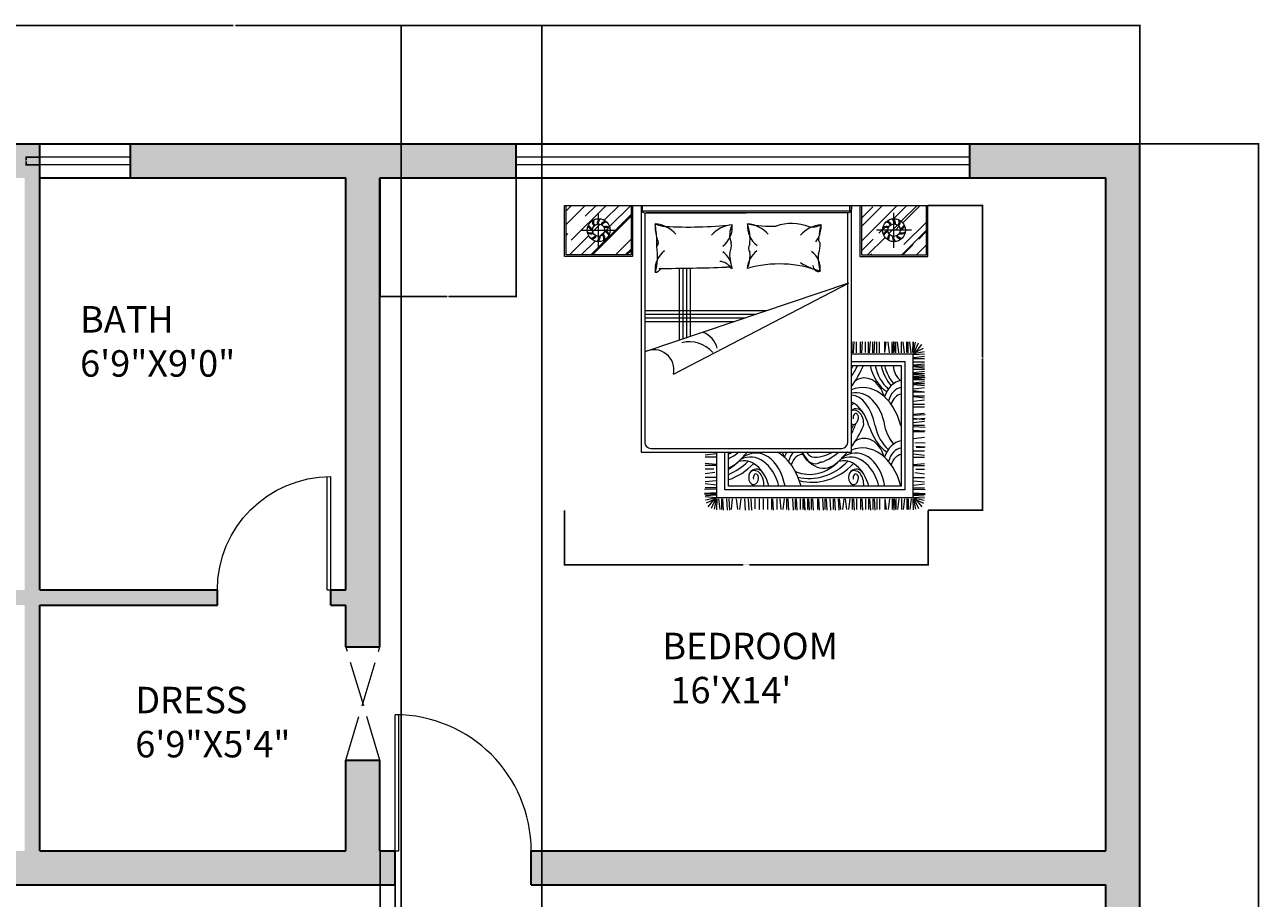
# Model space of a CAD drawing. Units: inches. Extents: x 1919 to 2461, y 2470 to 3159.
# Tile 6 of 6: x 2134 to 2461, y 2928 to 3159. Entities that reach past the tile are written whole.
import ezdxf

# ---------------------------------------------------------------- set-up
doc = ezdxf.new("R2010")
doc.units = ezdxf.units.IN
doc.linetypes.add('ACAD_ISO02W100', pattern=[15, 12, -3])
for name, color, linetype, lineweight in [('A-ANNO-DIMS', 2, 'Continuous', 18), ('A-AREA-IDEN', 7, 'Continuous', 18), ('A-DOOR', 3, 'Continuous', 18), ('A-FURN', 8, 'Continuous', 18), ('A-GLAZ', 4, 'Continuous', 18), ('A-WALL', 7, 'Continuous', 35), ('A-WALL-OVHD', 7, 'ACAD_ISO02W100', 13), ('A-WALL-PATT', 252, 'Continuous', 13)]:
    doc.layers.add(name, color=color, linetype=linetype, lineweight=lineweight)
doc.styles.get("Standard").update_dxf_attribs({"font": 'arial.ttf'})
doc.dimstyles.get("Standard").update_dxf_attribs({"dimtxt": 0.18, "dimasz": 0.18, "dimexe": 0.18, "dimexo": 0.0625, "dimgap": 0.09, "dimtad": 0, "dimtih": 1, "dimtoh": 1, "dimdec": 4, "dimzin": 0, "dimdsep": 46, "dimtxsty": 'Standard', "dimcen": 0.09, "dimadec": 0, "dimazin": 0, "dimtfac": 1, "dimtdec": 4, "dimtofl": 0, "dimtmove": 0, "dimatfit": 3, "dimfxl": 1, "dimtolj": 1, "dimtzin": 0, "dimarcsym": 0})

# ---------------------------------------------------------------- blocks, each defined once
blk = doc.blocks.new('A$C64B41DC1')
for p, q in [((0, 2.508), (2.99, 2.508)), ((0, 2.088), (0, 2.508)), ((0.012, 2.462), (0.058, 2.508)), ((0.012, 2.352), (0.168, 2.508)), ((0.012, 2.1), (0.012, 2.508)), ((0.054, 2.221), (0.341, 2.508)), ((0.169, 2.418), (0.259, 2.508)), ((0.28, 2.16), (0.28, 2.448)), ((0.327, 2.386), (0.448, 2.508)), ((0.37, 2.333), (0.545, 2.508)), ((0.548, 2.508), (0.548, 2.1)), ((0.56, 2.508), (0.56, 2.088)), ((0.63, 2.508), (0.63, 0.478)), ((0.64, 2.461), (0.64, 2.508)), ((0.64, 2.508), (2.344, 2.508)), ((2.344, 2.461), (0.64, 2.461)), ((0.66, 2.446), (1.495, 2.446)), ((0.66, 2.446), (0.66, 0.558)), ((1.495, 2.446), (0.67, 2.446)), ((2.33, 2.446), (1.495, 2.446)), ((2.33, 0.558), (2.33, 2.446)), ((2.344, 2.508), (2.36, 2.508)), ((2.344, 2.508), (2.344, 2.461)), ((2.36, 2.508), (2.36, 2.476)), ((2.36, 0.478), (2.36, 2.508)), ((2.43, 2.508), (2.43, 2.088)), ((2.442, 2.508), (2.442, 2.1)), ((2.442, 2.333), (2.617, 2.508)), ((2.442, 2.214), (2.736, 2.508)), ((2.442, 2.404), (2.535, 2.497)), ((2.705, 2.398), (2.815, 2.508)), ((2.71, 2.16), (2.71, 2.448)), ((2.769, 2.377), (2.9, 2.508)), ((2.782, 2.365), (2.925, 2.508)), ((2.978, 2.1), (2.978, 2.508)), ((2.99, 2.088), (2.99, 2.508)), ((0.216, 2.1), (0.548, 2.432)), ((0.23, 2.1), (0.548, 2.418)), ((0.231, 2.291), (0.294, 2.353)), ((2.667, 2.276), (2.738, 2.346)), ((2.791, 2.185), (2.978, 2.371)), ((0.012, 2.261), (0.027, 2.276)), ((0.04, 2.1), (0.198, 2.258)), ((0.136, 2.304), (0.425, 2.304)), ((0.291, 2.254), (0.33, 2.294)), ((0.341, 2.304), (0.36, 2.324)), ((2.492, 2.1), (2.637, 2.245)), ((2.854, 2.304), (2.566, 2.304)), ((2.585, 2.278), (2.616, 2.309)), ((2.616, 2.309), (2.631, 2.324)), ((2.725, 2.308), (2.751, 2.334)), ((2.775, 2.1), (2.978, 2.304)), ((2.914, 2.231), (2.978, 2.295)), ((0.137, 2.1), (0.251, 2.214)), ((0.419, 2.1), (0.548, 2.229)), ((0.499, 2.1), (0.548, 2.149)), ((0.513, 2.1), (0.548, 2.135)), ((2.442, 2.135), (2.538, 2.231)), ((2.783, 2.1), (2.868, 2.185)), ((2.896, 2.1), (2.978, 2.182)), ((0.56, 2.088), (0, 2.088)), ((0.548, 2.1), (0.012, 2.1)), ((2.43, 2.088), (2.99, 2.088)), ((2.442, 2.1), (2.978, 2.1)), ((2.517, 2.1), (2.527, 2.11)), ((0.942, 1.99), (0.942, 1.397)), ((0.972, 1.991), (0.972, 1.408)), ((1.002, 1.991), (1.002, 1.418)), ((1.032, 1.992), (1.032, 1.428)), ((2.335, 1.868), (0.661, 1.303)), ((0.896, 1.119), (2.335, 1.868)), ((1.664, 1.641), (0.66, 1.641)), ((1.575, 1.611), (0.66, 1.611)), ((2.366, 1.295), (2.366, 1.384)), ((2.377, 1.295), (2.382, 1.389)), ((2.403, 1.295), (2.403, 1.384)), ((2.435, 1.295), (2.435, 1.384)), ((2.445, 1.295), (2.45, 1.389)), ((2.477, 1.296), (2.477, 1.384)), ((2.5, 1.295), (2.5, 1.384)), ((2.51, 1.295), (2.516, 1.389)), ((2.537, 1.295), (2.537, 1.384)), ((2.547, 1.295), (2.552, 1.389)), ((2.568, 1.295), (2.568, 1.384)), ((2.592, 1.295), (2.592, 1.384)), ((2.635, 1.296), (2.635, 1.384)), ((2.636, 1.296), (2.647, 1.384)), ((2.673, 1.295), (2.662, 1.384)), ((2.694, 1.295), (2.694, 1.384)), ((2.704, 1.295), (2.71, 1.389)), ((2.713, 1.296), (2.723, 1.384)), ((2.725, 1.295), (2.725, 1.384)), ((2.749, 1.295), (2.739, 1.384)), ((2.772, 1.295), (2.772, 1.384)), ((2.796, 1.295), (2.785, 1.384)), ((2.815, 1.296), (2.815, 1.384)), ((2.815, 1.296), (2.815, 1.384)), ((2.828, 1.295), (2.828, 1.384)), ((2.828, 1.295), (2.828, 1.384)), ((2.852, 1.295), (2.842, 1.384)), ((2.852, 1.295), (2.842, 1.384)), ((2.865, 1.297), (2.869, 1.386)), ((2.871, 1.296), (2.871, 1.384)), ((2.871, 1.296), (2.888, 1.382)), ((2.871, 1.293), (2.954, 1.332)), ((2.877, 1.296), (2.913, 1.376)), ((2.889, 1.301), (2.939, 1.364)), ((2.36, 1.287), (2.864, 1.287)), ((2.36, 1.223), (2.8, 1.223)), ((2.8, 1.223), (2.8, 0.166)), ((2.864, 1.287), (2.864, 0.102)), ((2.872, 1.288), (2.959, 1.306)), ((2.872, 1.256), (2.96, 1.267)), ((2.872, 1.249), (2.96, 1.249)), ((2.872, 1.221), (2.96, 1.221)), ((2.874, 1.282), (2.96, 1.287)), ((2.36, 1.191), (2.768, 1.191)), ((2.768, 1.191), (2.768, 0.198)), ((2.872, 1.195), (2.96, 1.205)), ((2.872, 1.187), (2.96, 1.187)), ((2.872, 1.181), (2.96, 1.171)), ((2.872, 1.159), (2.96, 1.159)), ((2.872, 1.133), (2.96, 1.143)), ((2.872, 1.125), (2.96, 1.125)), ((2.872, 1.119), (2.96, 1.109)), ((2.872, 1.104), (2.96, 1.093)), ((2.872, 1.097), (2.96, 1.097)), ((2.872, 1.086), (2.966, 1.091)), ((2.872, 1.086), (2.96, 1.075)), ((2.872, 1.076), (2.96, 1.076)), ((2.872, 1.049), (2.96, 1.06)), ((2.872, 1.042), (2.96, 1.042)), ((2.872, 1.035), (2.96, 1.025)), ((2.872, 0.999), (2.96, 1.009)), ((2.872, 0.985), (2.96, 0.974)), ((2.872, 0.973), (2.96, 0.973)), ((2.872, 0.941), (2.96, 0.941)), ((2.872, 0.935), (2.96, 0.924)), ((2.872, 0.898), (2.96, 0.908)), ((2.872, 0.873), (2.96, 0.873)), ((2.872, 0.85), (2.96, 0.85)), ((2.872, 0.789), (2.96, 0.799)), ((2.872, 0.782), (2.966, 0.787)), ((2.872, 0.757), (2.96, 0.747)), ((2.872, 0.75), (2.966, 0.756)), ((2.872, 0.72), (2.96, 0.731)), ((2.872, 0.699), (2.96, 0.699)), ((2.872, 0.689), (2.966, 0.684)), ((2.872, 0.658), (2.966, 0.652)), ((2.872, 0.647), (2.96, 0.647)), ((2.872, 0.59), (2.96, 0.601)), ((2.882, 0.558), (2.966, 0.554)), ((2.891, 0.526), (2.966, 0.522)), ((2.893, 0.517), (2.96, 0.517)), ((0.63, 0.478), (2.36, 0.478)), ((0.71, 0.508), (2.28, 0.508)), ((1.246, 0.463), (1.158, 0.452)), ((1.246, 0.437), (1.158, 0.437)), ((1.254, 0.102), (1.254, 0.478)), ((1.318, 0.166), (1.318, 0.478)), ((1.35, 0.198), (1.35, 0.478)), ((2.872, 0.488), (2.96, 0.488)), ((2.872, 0.463), (2.96, 0.452)), ((2.872, 0.437), (2.96, 0.437)), ((1.246, 0.375), (1.158, 0.385)), ((1.246, 0.368), (1.158, 0.368)), ((1.229, 0.336), (1.158, 0.336)), ((1.235, 0.309), (1.158, 0.3)), ((2.872, 0.375), (2.96, 0.385)), ((2.872, 0.368), (2.96, 0.368)), ((2.883, 0.309), (2.96, 0.3)), ((2.89, 0.336), (2.96, 0.336)), ((1.246, 0.268), (1.158, 0.268)), ((1.246, 0.242), (1.158, 0.232)), ((1.246, 0.206), (1.158, 0.216)), ((2.872, 0.268), (2.96, 0.268)), ((2.872, 0.242), (2.96, 0.232)), ((2.872, 0.206), (2.96, 0.216)), ((1.246, 0.174), (1.152, 0.169)), ((1.246, 0.143), (1.152, 0.138)), ((1.246, 0.133), (1.152, 0.128)), ((1.246, 0.185), (1.158, 0.185)), ((1.246, 0.132), (1.158, 0.132)), ((1.246, 0.132), (1.158, 0.132)), ((1.246, 0.1), (1.158, 0.11)), ((1.246, 0.123), (1.159, 0.117)), ((2.864, 0.102), (1.254, 0.102)), ((2.8, 0.166), (1.318, 0.166)), ((2.768, 0.198), (1.35, 0.198)), ((2.872, 0.185), (2.96, 0.185)), ((2.872, 0.174), (2.966, 0.169)), ((2.872, 0.143), (2.966, 0.138)), ((2.872, 0.133), (2.966, 0.128)), ((2.872, 0.132), (2.96, 0.132)), ((2.872, 0.123), (2.959, 0.117)), ((2.874, 0.107), (2.96, 0.102)), ((1.246, 0.101), (1.159, 0.083)), ((1.247, 0.096), (1.164, 0.058)), ((1.229, 0.088), (1.179, 0.026)), ((1.242, 0.093), (1.205, 0.013)), ((1.247, 0.093), (1.231, 0.007)), ((1.253, 0.092), (1.249, 0.003)), ((1.266, 0.094), (1.276, 0.005)), ((1.29, 0.094), (1.29, 0.005)), ((1.3, 0.094), (1.305, 0)), ((1.331, 0.094), (1.337, 0)), ((1.352, 0.094), (1.358, 0)), ((1.38, 0.094), (1.37, 0.005)), ((1.412, 0.093), (1.422, 0.005)), ((1.449, 0.094), (1.438, 0.005)), ((1.48, 0.094), (1.485, 0)), ((1.511, 0.094), (1.517, 0)), ((1.532, 0.094), (1.538, 0)), ((1.564, 0.094), (1.564, 0.01)), ((1.602, 0.094), (1.602, 0.005)), ((1.634, 0.094), (1.634, 0.005)), ((1.67, 0.094), (1.67, 0.005)), ((1.702, 0.094), (1.702, 0.005)), ((1.712, 0.094), (1.717, 0)), ((1.745, 0.093), (1.745, 0.005)), ((1.77, 0.093), (1.78, 0.005)), ((1.806, 0.094), (1.796, 0.005)), ((1.827, 0.094), (1.827, 0.005)), ((1.838, 0.094), (1.843, 0)), ((1.875, 0.094), (1.88, 0)), ((1.896, 0.094), (1.896, 0.005)), ((1.906, 0.094), (1.911, 0)), ((1.938, 0.093), (1.938, 0.005)), ((1.961, 0.094), (1.961, 0.005)), ((1.964, 0.093), (1.974, 0.005)), ((1.971, 0.094), (1.977, 0)), ((1.998, 0.094), (1.998, 0.005)), ((2.008, 0.094), (2.013, 0)), ((2.029, 0.094), (2.029, 0.005)), ((2.039, 0.094), (2.045, 0)), ((2.08, 0.094), (2.08, 0.005)), ((2.09, 0.094), (2.095, 0)), ((2.122, 0.094), (2.127, 0)), ((2.141, 0.094), (2.141, 0.005)), ((2.152, 0.094), (2.157, 0)), ((2.183, 0.094), (2.188, 0)), ((2.209, 0.094), (2.209, 0.005)), ((2.22, 0.094), (2.225, 0)), ((2.251, 0.094), (2.256, 0)), ((2.26, 0.093), (2.271, 0.005)), ((2.297, 0.094), (2.286, 0.005)), ((2.309, 0.093), (2.319, 0.005)), ((2.346, 0.094), (2.335, 0.005)), ((2.366, 0.094), (2.366, 0.005)), ((2.377, 0.094), (2.382, 0)), ((2.403, 0.094), (2.403, 0.005)), ((2.435, 0.094), (2.435, 0.005)), ((2.445, 0.094), (2.45, 0)), ((2.477, 0.093), (2.477, 0.005)), ((2.5, 0.094), (2.5, 0.005)), ((2.51, 0.094), (2.516, 0)), ((2.537, 0.094), (2.537, 0.005)), ((2.547, 0.094), (2.552, 0)), ((2.568, 0.094), (2.568, 0.005)), ((2.592, 0.094), (2.592, 0.005)), ((2.635, 0.093), (2.635, 0.005)), ((2.636, 0.093), (2.647, 0.005)), ((2.673, 0.094), (2.662, 0.005)), ((2.694, 0.094), (2.694, 0.005)), ((2.704, 0.094), (2.71, 0)), ((2.713, 0.093), (2.723, 0.005)), ((2.725, 0.094), (2.725, 0.005)), ((2.749, 0.094), (2.739, 0.005)), ((2.772, 0.094), (2.772, 0.005)), ((2.796, 0.094), (2.785, 0.005)), ((2.815, 0.093), (2.815, 0.005)), ((2.828, 0.094), (2.828, 0.005)), ((2.852, 0.094), (2.842, 0.005)), ((2.865, 0.092), (2.869, 0.003)), ((2.871, 0.096), (2.954, 0.058)), ((2.871, 0.093), (2.888, 0.007)), ((2.872, 0.101), (2.959, 0.083)), ((2.877, 0.093), (2.913, 0.013)), ((2.889, 0.088), (2.939, 0.026))]:
    blk.add_line(p, q)
at = {"ltscale": 10}
for p, q in [((1.486, 1.581), (0.66, 1.581)), ((1.397, 1.551), (0.66, 1.551))]:
    blk.add_line(p, q, dxfattribs=at)
for centre, radius in [((0.28, 2.304), 0.0942), ((0.28, 2.304), 0.051), ((2.71, 2.304), 0.0942), ((2.71, 2.304), 0.051)]:
    blk.add_circle(centre, radius)
for centre, radius, start, end in [((0.66, 2.476), 0.03, 180, 270), ((2.33, 2.476), 0.03, 270, 0), ((0.246, 2.366), 0.0605, 208.17, 254.4897), ((0.242, 2.361), 0.0462, 196.3002, 256.538), ((0.289, 2.374), 0.0605, 172.17, 218.4897), ((0.283, 2.373), 0.0462, 160.3002, 220.538), ((0.329, 2.356), 0.0605, 136.17, 182.4897), ((0.323, 2.358), 0.0462, 124.3002, 184.538), ((0.35, 2.318), 0.0605, 100.17, 146.4897), ((0.347, 2.323), 0.0462, 88.3002, 148.538), ((1.053, 2.33), 0.308, 175.3048, 198.6942), ((-0.87, 2.094), 1.636, 4.8098, 9.1892), ((0.858, 2.628), 0.295, 247.5179, 264.267), ((0.728, 2.111), 0.245, 40.4189, 85.9871), ((1.016, 5.71), 3.38, 266.8134, 276.1602), ((1.396, 2.104), 0.245, 94.0129, 139.5811), ((1.186, 2.329), 0.194, 306.5711, 5.89), ((1.535, 2.265), 0.177, 151.7736, 201.6983), ((1.699, 2.335), 0.194, 174.11, 233.4289), ((1.148, 2.231), 0.378, 353.4947, 19.1867), ((1.687, 3.192), 0.856, 257.7438, 273.6284), ((1.488, 2.111), 0.245, 40.4189, 85.9871), ((1.867, 1.971), 0.388, 68.2026, 108.9817), ((2.127, 2.104), 0.245, 94.0129, 139.5811), ((2.034, 2.486), 0.156, 261.5958, 298.9092), ((1.916, 2.329), 0.194, 333.7371, 5.89), ((2.606, 2.203), 0.517, 163.6046, 172.3273), ((2.643, 2.323), 0.0462, 31.462, 91.6998), ((2.64, 2.318), 0.0605, 33.5103, 79.83), ((2.667, 2.358), 0.0462, 355.462, 55.6998), ((2.662, 2.356), 0.0605, 357.5103, 43.83), ((2.707, 2.373), 0.0462, 319.462, 19.6998), ((2.702, 2.374), 0.0605, 321.5103, 7.83), ((2.749, 2.361), 0.0462, 283.462, 343.6998), ((2.745, 2.366), 0.0605, 285.5103, 331.83), ((0.215, 2.328), 0.0462, 232.3002, 292.538), ((0.216, 2.334), 0.0605, 244.17, 290.4897), ((0.214, 2.285), 0.0462, 268.3002, 328.538), ((0.211, 2.29), 0.0605, 280.17, 326.4897), ((0.238, 2.249), 0.0462, 304.3002, 4.538), ((0.232, 2.252), 0.0605, 316.17, 2.4897), ((0.278, 2.235), 0.0462, 340.3002, 40.538), ((0.272, 2.233), 0.0605, 352.17, 38.4897), ((0.345, 2.274), 0.0605, 64.17, 110.4897), ((0.345, 2.28), 0.0462, 52.3002, 112.538), ((0.319, 2.246), 0.0462, 16.3002, 76.538), ((0.315, 2.242), 0.0605, 28.17, 74.4897), ((1.916, 2.329), 0.194, 320.9404, 333.7371), ((2.135, 2.231), 0.0459, 165.3506, 223.2684), ((2.645, 2.28), 0.0462, 67.462, 127.6998), ((2.645, 2.274), 0.0605, 69.5103, 115.83), ((2.675, 2.242), 0.0605, 105.5103, 151.83), ((2.671, 2.246), 0.0462, 103.462, 163.6998), ((2.718, 2.233), 0.0605, 141.5103, 187.83), ((2.712, 2.235), 0.0462, 139.462, 199.6998), ((2.758, 2.252), 0.0605, 177.5103, 223.83), ((2.753, 2.249), 0.0462, 175.462, 235.6998), ((2.78, 2.29), 0.0605, 213.5103, 259.83), ((2.777, 2.285), 0.0462, 211.462, 271.6998), ((2.774, 2.334), 0.0605, 249.5103, 295.83), ((2.775, 2.328), 0.0462, 247.462, 307.6998), ((0.938, 1.978), 0.194, 126.5711, 185.89), ((0.269, 2.094), 0.496, 344.0243, 8.7071), ((0.727, 2.201), 0.0446, 314.4736, 42.1713), ((-1.601, 2.277), 2.362, 357.3905, 358.8876), ((1.204, 2.178), 0.168, 337.017, 7.5368), ((1.706, 1.971), 0.204, 127.1197, 175.09), ((1.567, 2.155), 0.0547, 142.0833, 220.902), ((1.935, 2.178), 0.168, 337.017, 7.5368), ((1.269, 1.925), 0.122, 33.628, 86.4744), ((1.186, 1.971), 0.194, 4.3181, 53.4289), ((1.541, 2.097), 0.183, 175.2233, 196.23), ((1.196, 2.098), 0.33, 343.7954, 3.5554), ((2.275, 2.579), 0.637, 238.3499, 254.3137), ((1.939, 1.991), 0.165, 351.2621, 55.7572), ((2.462, 2.072), 0.375, 173.8296, 196.4356), ((0.742, 2.015), 0.057, 273.4709, 328.5412), ((0.728, 2.202), 0.245, 274.0129, 278.3417), ((0.725, 18.844), 16.855, 270.174, 272.0521), ((1.34, 1.94), 0.0603, 49.0991, 101.3702), ((1.768, 1.063), 0.963, 69.6507, 105.9631), ((2.091, 2.012), 0.0478, 179.7727, 283.8018), ((1.075, 1.287), 0.187, 14.1863, 69.1212), ((1.027, 1.133), 0.253, 40.629, 104.3712), ((0.735, 1.155), 0.165, 347.3109, 116.4454), ((0.71, 0.558), 0.05, 180, 270), ((2.28, 0.558), 0.05, 270, 0)]:
    blk.add_arc(centre, radius, start, end)
for centre, major_axis, ratio, start_param, end_param in [((1.994, 1.626), (0, -0.753), 0.68, 0.797284, 0.954936), ((2.064, 1.466), (0, -0.532), 0.68, 7.239912, 7.311536), ((1.905, 1.74), (0, -0.984), 0.68, 0.74745, 0.979724), ((2.467, 0.822), (0, -0.266), 0.68, 2.006169, 3.565187), ((2.746, 1.308), (0, 0.361), 0.68, 1.900046, 2.742661), ((2.787, 1.308), (0, 0.361), 0.68, 1.900046, 2.614747), ((2.837, 1.308), (0, 0.361), 0.68, 1.900046, 2.479658), ((2.861, 1.321), (0, 0.361), 0.68, 1.938265, 2.479658), ((2.806, 1.208), (0, -0.152), 0.68, 4.821745, 5.895886), ((2.451, 0.507), (0, 0.502), 0.68, 5.095327, 6.553458), ((2.786, 0.807), (0, -0.261), 0.68, 3.244645, 4.205018), ((2.396, 0.603), (0, 0.364), 0.68, -1.3172, 0.145284), ((2.351, 0.564), (0.007, 0.382), 0.56205, -1.21172, -0.009991), ((2.778, 0.829), (0, -0.18), 0.68, 3.227058, 4.318474), ((2.782, 0.797), (0, -0.159), 0.68, 3.272942, 4.229533), ((2.296, 0.577), (0, -0.326), 0.68, 1.938944, 2.850232), ((2.04, 1.601), (0, -0.876), 0.68, 6.849801, 6.887077), ((2.4, 0.713), (0, -0.121), 0.68, 2.284368, 3.652258), ((2.383, 0.708), (0, 0.115), 0.68, 4.593909, 6.585576), ((2.377, 0.765), (0, -0.0593), 0.68, 5.841311, 7.755362), ((1.994, 1.13), (-0.068, 0.744), 0.610498, 3.917146, 4.063997), ((2.396, 0.763), (0, -0.0317), 0.68, 1.462497, 5.046281), ((2.064, 0.969), (0, -0.532), 0.68, 7.239912, 7.336618), ((1.905, 1.243), (0, -0.984), 0.68, 0.74745, 0.979724), ((2.467, 0.325), (0, -0.266), 0.68, 2.006169, 3.565187), ((2.746, 0.811), (-0.06, 0.373), 0.695517, 1.775813, 2.548612), ((2.787, 0.811), (0, 0.361), 0.68, 1.900046, 2.614747), ((2.861, 0.824), (0, 0.361), 0.68, 1.938265, 2.479658), ((2.451, 0.01), (0, 0.502), 0.68, 5.095327, 6.553458), ((2.786, 0.31), (0, -0.261), 0.68, 3.244645, 4.205018), ((2.778, 0.332), (0, -0.18), 0.68, 3.227058, 4.318474), ((1.242, 0.969), (0, -0.532), 0.68, 6.586764, 6.677612), ((1.171, 1.13), (-0.116, 0.724), 0.59432, 3.291697, 3.50733), ((1.193, 0.918), (0, -0.624), 0.68, 0.378672, 0.625379), ((1.309, 0.66), (0, -0.315), 0.68, 6.475719, 6.949396), ((1.474, 0.08), (0, -0.326), 0.68, 1.938944, 3.339184), ((1.083, 1.243), (0, -0.984), 0.68, 0.565948, 0.680366), ((1.528, 0.067), (0, -0.37), 0.68, 1.930561, 3.464283), ((1.574, 0.106), (0, 0.364), 0.68, -1.3172, 0.476403), ((1.629, 0.01), (0, 0.502), 0.68, 6.655152, 6.661293), ((1.629, 0.01), (0, 0.502), 0.68, 5.095327, 5.911219), ((1.644, 0.325), (0, -0.266), 0.68, 2.006169, 2.182797), ((1.964, 0.31), (0, -0.261), 0.68, 4.015924, 4.205018), ((1.956, 0.332), (0, -0.18), 0.68, 3.770744, 4.318474), ((1.96, 0.3), (0, -0.159), 0.68, 3.14258, 4.229533), ((2.016, 0.918), (0, -0.624), 0.68, -0.280078, 0.625379), ((2.061, 0.562), (0, -0.18), 0.68, 5.194792, 5.929328), ((2.061, 0.562), (0, -0.18), 0.68, 5.194792, 6.723255), ((2.131, 0.66), (0, -0.315), 0.68, 5.328638, 6.949396), ((2.055, 0.566), (0, -0.13), 0.68, 5.450951, 6.054641), ((2.064, 0.969), (0, -0.532), 0.68, 6.20013, 6.677612), ((1.994, 1.13), (-0.068, 0.744), 0.610498, 3.199135, 3.592282), ((2.296, 0.08), (0, -0.326), 0.68, 1.938944, 3.339184), ((1.905, 1.243), (0, -0.984), 0.68, 0.565948, 0.680366), ((2.351, 0.067), (0, -0.37), 0.68, 1.930561, 3.464283), ((2.396, 0.106), (0, 0.364), 0.68, -1.3172, 0.476403), ((2.451, 0.01), (0, 0.502), 0.68, 6.655152, 6.661293), ((2.782, 0.3), (0, -0.159), 0.68, 3.272942, 4.229533), ((1.191, 1.107), (0, 0.846), 0.68, 3.421828, 3.728616), ((1.218, 1.105), (0, -0.876), 0.68, 6.507006, 6.887077), ((1.555, 0.269), (0, -0.0593), 0.68, 3.732151, 7.755362), ((1.578, 0.217), (0, -0.121), 0.68, 2.284368, 3.726131), ((1.561, 0.211), (0, 0.115), 0.68, 4.593909, 6.647252), ((2.013, 1.107), (0, 0.846), 0.68, 2.978727, 3.728616), ((2.04, 1.105), (0, -0.876), 0.68, 6.099302, 6.887077), ((2.377, 0.269), (0, -0.0593), 0.68, 3.732151, 7.755362), ((2.4, 0.217), (0, -0.121), 0.68, 2.284368, 3.726131), ((2.383, 0.211), (0, 0.115), 0.68, 4.593909, 6.647252), ((1.574, 0.266), (0, -0.0317), 0.68, 1.462497, 5.046281), ((2.396, 0.266), (0, -0.0317), 0.68, 1.462497, 5.046281)]:
    blk.add_ellipse(centre, major_axis=major_axis, ratio=ratio, start_param=start_param, end_param=end_param)
blk = doc.blocks.new('DOOR-SGL-30IN')
for p, q in [((0, 0), (0, 30)), ((1, 0), (1, 29.98)), ((1, 0), (0, 0))]:
    blk.add_line(p, q)
blk.add_arc((0, 0), 30, 0, 90)
blk = doc.blocks.new('DOOR-SGL-36IN')
for p, q in [((0, 0), (-36, 0)), ((0, 1), (-35.99, 1)), ((0, 0), (0, 1))]:
    blk.add_line(p, q)
blk.add_arc((0, 0), 36, 90, 180)
blk = doc.blocks.new('WIN-GLAZ-120IN')
for p, q in [((120, 0), (0, 0)), ((120, -2), (0, -2))]:
    blk.add_line(p, q)
blk = doc.blocks.new('WIN-GLAZ-24IN')
for p, q in [((-2, 24), (-2, 0)), ((0, 24), (0, 0))]:
    blk.add_line(p, q)
blk = doc.blocks.new('OPENING-OVHD-30IN')
for p, q in [((0, 0), (9, 30)), ((9, 0), (0, 30))]:
    blk.add_line(p, q)
blk = doc.blocks.new('*D9')
at = {"layer": 'A-ANNO-DIMS', "color": 0, "lineweight": -2, "transparency": 16777216}
for p, q in [((2277.14, 3030.73), (2277.14, 3016.19)), ((2373.26, 3030.73), (2373.26, 3016.19)), ((2277.32, 3016.37), (2324.38, 3016.37)), ((2373.08, 3016.37), (2326.01, 3016.37))]:
    blk.add_line(p, q, dxfattribs=at)
at = {"layer": 'A-ANNO-DIMS', "color": 0, "transparency": 16777216}
for points in [[(2277.32, 3016.4), (2277.32, 3016.34), (2277.14, 3016.37)], [(2373.08, 3016.4), (2373.08, 3016.34), (2373.26, 3016.37)]]:
    blk.add_solid(points, dxfattribs=at)
at = {"layer": 'Defpoints', "color": 0, "transparency": 16777216}
for p in [(2277.14, 3030.79), (2373.26, 3030.79), (2373.26, 3016.37)]:
    blk.add_point(p, dxfattribs=at)
at = {"layer": 'A-ANNO-DIMS', "color": 0, "transparency": 16777216, "insert": (2325.2, 3016.37), "char_height": 0.18, "attachment_point": 5}
blk.add_mtext('\\A1;BED 96 TYP.', dxfattribs=at)
blk = doc.blocks.new('*D10')
at = {"layer": 'A-ANNO-DIMS', "color": 0, "lineweight": -2, "transparency": 16777216}
for p, q in [((2373.32, 3111.41), (2387.85, 3111.41)), ((2387.67, 3111.23), (2387.67, 3071.28)), ((2387.67, 3030.97), (2387.67, 3070.92)), ((2373.32, 3030.79), (2387.85, 3030.79))]:
    blk.add_line(p, q, dxfattribs=at)
at = {"layer": 'A-ANNO-DIMS', "color": 0, "transparency": 16777216}
for points in [[(2387.64, 3111.23), (2387.7, 3111.23), (2387.67, 3111.41)], [(2387.64, 3030.97), (2387.7, 3030.97), (2387.67, 3030.79)]]:
    blk.add_solid(points, dxfattribs=at)
at = {"layer": 'Defpoints', "color": 0, "transparency": 16777216}
for p in [(2373.26, 3111.41), (2387.67, 3111.41), (2373.26, 3030.79)]:
    blk.add_point(p, dxfattribs=at)
at = {"layer": 'A-ANNO-DIMS', "color": 0, "transparency": 16777216, "insert": (2387.67, 3071.1), "char_height": 0.18, "attachment_point": 5}
blk.add_mtext('\\A1;81 TYP.', dxfattribs=at)
blk = doc.blocks.new('*D19')
at = {"layer": 'A-ANNO-DIMS', "color": 0, "lineweight": -2, "transparency": 16777216}
for p, q in [((2138.32, 3122.11), (2138.32, 3118.39)), ((2162.32, 3122.11), (2162.32, 3118.39)), ((2138.5, 3118.57), (2149.2, 3118.57)), ((2162.14, 3118.57), (2151.43, 3118.57))]:
    blk.add_line(p, q, dxfattribs=at)
at = {"layer": 'A-ANNO-DIMS', "color": 0, "transparency": 16777216}
for points in [[(2138.5, 3118.6), (2138.5, 3118.54), (2138.32, 3118.57)], [(2162.14, 3118.6), (2162.14, 3118.54), (2162.32, 3118.57)]]:
    blk.add_solid(points, dxfattribs=at)
at = {"layer": 'Defpoints', "color": 0, "transparency": 16777216}
for p in [(2138.32, 3122.17), (2162.32, 3122.17), (2162.32, 3118.57)]:
    blk.add_point(p, dxfattribs=at)
at = {"layer": 'A-ANNO-DIMS', "color": 0, "transparency": 16777216, "insert": (2150.32, 3118.57), "char_height": 0.18, "attachment_point": 5}
blk.add_mtext('\\A1;WINDOW 24 TYP.', dxfattribs=at)
blk = doc.blocks.new('*D20')
at = {"layer": 'A-ANNO-DIMS', "color": 0, "lineweight": -2, "transparency": 16777216}
for p, q in [((2138.25, 3124.17), (2134.54, 3124.17)), ((2138.25, 3122.17), (2134.54, 3122.17)), ((2134.72, 3123.99), (2134.72, 3123.35)), ((2134.72, 3122.35), (2134.72, 3122.99))]:
    blk.add_line(p, q, dxfattribs=at)
at = {"layer": 'A-ANNO-DIMS', "color": 0, "transparency": 16777216}
for points in [[(2134.69, 3123.99), (2134.75, 3123.99), (2134.72, 3124.17)], [(2134.69, 3122.35), (2134.75, 3122.35), (2134.72, 3122.17)]]:
    blk.add_solid(points, dxfattribs=at)
at = {"layer": 'Defpoints', "color": 0, "transparency": 16777216}
for p in [(2134.72, 3122.17), (2138.32, 3124.17), (2138.32, 3122.17)]:
    blk.add_point(p, dxfattribs=at)
at = {"layer": 'A-ANNO-DIMS', "color": 0, "transparency": 16777216, "insert": (2134.72, 3123.17), "char_height": 0.18, "attachment_point": 5}
blk.add_mtext('\\A1;2 TYP.', dxfattribs=at)
blk = doc.blocks.new('*D23')
at = {"layer": 'A-ANNO-DIMS', "color": 0, "lineweight": -2, "transparency": 16777216}
for p, q in [((1950.32, 3072.73), (1950.32, 3159.21)), ((1950.5, 3159.03), (2189.52, 3159.03)), ((2429.14, 3159.03), (2190.11, 3159.03)), ((2429.32, 3127.73), (2429.32, 3159.21))]:
    blk.add_line(p, q, dxfattribs=at)
at = {"layer": 'A-ANNO-DIMS', "color": 0, "transparency": 16777216}
for points in [[(1950.5, 3159.06), (1950.5, 3159), (1950.32, 3159.03)], [(2429.14, 3159.06), (2429.14, 3159), (2429.32, 3159.03)]]:
    blk.add_solid(points, dxfattribs=at)
at = {"layer": 'Defpoints', "color": 0, "transparency": 16777216}
for p in [(2429.32, 3159.03), (2429.32, 3127.67), (1950.32, 3072.67)]:
    blk.add_point(p, dxfattribs=at)
at = {"layer": 'A-ANNO-DIMS', "color": 0, "transparency": 16777216, "insert": (2189.82, 3159.03), "char_height": 0.18, "attachment_point": 5}
blk.add_mtext('\\A1;479', dxfattribs=at)
blk = doc.blocks.new('*D27')
at = {"layer": 'A-ANNO-DIMS', "color": 0, "lineweight": -2, "transparency": 16777216}
for p, q in [((2228.32, 3118.61), (2228.32, 3087.14)), ((2264.32, 3118.61), (2264.32, 3087.14)), ((2228.5, 3087.32), (2246.1, 3087.32)), ((2264.14, 3087.32), (2246.53, 3087.32))]:
    blk.add_line(p, q, dxfattribs=at)
at = {"layer": 'A-ANNO-DIMS', "color": 0, "transparency": 16777216}
for points in [[(2228.5, 3087.35), (2228.5, 3087.29), (2228.32, 3087.32)], [(2264.14, 3087.35), (2264.14, 3087.29), (2264.32, 3087.32)]]:
    blk.add_solid(points, dxfattribs=at)
at = {"layer": 'Defpoints', "color": 0, "transparency": 16777216}
for p in [(2228.32, 3118.67), (2264.32, 3118.67), (2228.32, 3087.32)]:
    blk.add_point(p, dxfattribs=at)
at = {"layer": 'A-ANNO-DIMS', "color": 0, "transparency": 16777216, "insert": (2246.32, 3087.32), "char_height": 0.18, "attachment_point": 5}
blk.add_mtext('\\A1;36', dxfattribs=at)
blk = doc.blocks.new('*D36')
at = {"layer": 'A-ANNO-DIMS', "color": 0, "lineweight": -2, "transparency": 16777216}
for p, q in [((2429.38, 3127.67), (2460.85, 3127.67)), ((2460.67, 3127.49), (2460.67, 2923.35)), ((2460.67, 2718.85), (2460.67, 2922.99)), ((2429.38, 2718.67), (2460.85, 2718.67))]:
    blk.add_line(p, q, dxfattribs=at)
at = {"layer": 'A-ANNO-DIMS', "color": 0, "transparency": 16777216}
for points in [[(2460.64, 3127.49), (2460.7, 3127.49), (2460.67, 3127.67)], [(2460.64, 2718.85), (2460.7, 2718.85), (2460.67, 2718.67)]]:
    blk.add_solid(points, dxfattribs=at)
at = {"layer": 'Defpoints', "color": 0, "transparency": 16777216}
for p in [(2429.32, 3127.67), (2460.67, 3127.67), (2429.32, 2718.67)]:
    blk.add_point(p, dxfattribs=at)
at = {"layer": 'A-ANNO-DIMS', "color": 0, "transparency": 16777216, "insert": (2460.67, 2923.17), "char_height": 0.18, "attachment_point": 5}
blk.add_mtext('\\A1;409', dxfattribs=at)
blk = doc.blocks.new('*D42')
at = {"layer": 'A-ANNO-DIMS', "color": 0, "lineweight": -2, "transparency": 16777216}
for p, q in [((2233.88, 2630.46), (2233.88, 3159.21)), ((2234.06, 3159.03), (2252.1, 3159.03)), ((2270.93, 3159.03), (2252.89, 3159.03)), ((2271.11, 2661.64), (2271.11, 3159.21))]:
    blk.add_line(p, q, dxfattribs=at)
at = {"layer": 'A-ANNO-DIMS', "color": 0, "transparency": 16777216}
for points in [[(2234.06, 3159.06), (2234.06, 3159), (2233.88, 3159.03)], [(2270.93, 3159.06), (2270.93, 3159), (2271.11, 3159.03)]]:
    blk.add_solid(points, dxfattribs=at)
at = {"layer": 'Defpoints', "color": 0, "transparency": 16777216}
for p in [(2271.11, 3159.03), (2271.11, 2661.57), (2233.88, 2630.39)]:
    blk.add_point(p, dxfattribs=at)
at = {"layer": 'A-ANNO-DIMS', "color": 0, "transparency": 16777216, "insert": (2252.49, 3159.03), "char_height": 0.18, "attachment_point": 5}
blk.add_mtext('\\A1;37.23', dxfattribs=at)
blk = doc.blocks.new('*D43')
at = {"layer": 'A-ANNO-DIMS', "color": 0, "lineweight": -2, "transparency": 16777216}
for p, q in [((2228.32, 2940.61), (2228.32, 2470.14)), ((2232.32, 2940.61), (2232.32, 2470.14)), ((2228.5, 2470.32), (2230.16, 2470.32)), ((2232.14, 2470.32), (2230.47, 2470.32))]:
    blk.add_line(p, q, dxfattribs=at)
at = {"layer": 'A-ANNO-DIMS', "color": 0, "transparency": 16777216}
for points in [[(2228.5, 2470.35), (2228.5, 2470.29), (2228.32, 2470.32)], [(2232.14, 2470.35), (2232.14, 2470.29), (2232.32, 2470.32)]]:
    blk.add_solid(points, dxfattribs=at)
at = {"layer": 'Defpoints', "color": 0, "transparency": 16777216}
for p in [(2228.32, 2940.67), (2232.32, 2940.67), (2232.32, 2470.32)]:
    blk.add_point(p, dxfattribs=at)
at = {"layer": 'A-ANNO-DIMS', "color": 0, "transparency": 16777216, "insert": (2230.32, 2470.32), "char_height": 0.18, "attachment_point": 5}
blk.add_mtext('\\A1;4', dxfattribs=at)

msp = doc.modelspace()

# ---------------------------------------------------------------- hatches: boundary and pattern name
at = {"layer": 'A-WALL-PATT'}
h = msp.add_hatch(color=256, dxfattribs=at)
h.dxf.hatch_style = 1
h.paths.add_polyline_path([(1959.315, 2931.672), (2066.315, 2931.672), (2066.315, 2940.672), (2062.315, 2940.672), (2062.315, 3005.672), (2066.315, 3005.672), (2066.315, 3009.672), (2062.315, 3009.672), (2062.315, 3118.672), (2062.315, 3127.672), (2004.315, 3127.672), (2004.315, 3072.672), (1950.315, 3072.672), (1950.315, 3059.672), (1959.315, 3059.672), (1959.315, 3063.672), (2017.315, 3063.672), (2017.315, 3067.672), (2013.315, 3067.672), (2013.315, 3118.672), (2058.315, 3118.672), (2058.315, 3067.672), (2047.315, 3067.672), (2047.315, 3063.672), (2058.315, 3063.672), (2058.315, 2940.672), (1959.315, 2940.672), (1959.315, 2952.172), (1950.315, 2952.172), (1950.315, 2901.672), (1959.315, 2901.672)])
h.paths.add_polyline_path([(2120.315, 2791.672), (2145.315, 2791.672), (2145.315, 2795.672), (2124.315, 2795.672), (2124.315, 2803.3999), (2115.315, 2803.3999), (2115.315, 2799.3999), (2067.5871, 2751.672), (1959.315, 2751.672), (1959.315, 2781.672), (1950.315, 2781.672), (1950.315, 2718.672), (1959.315, 2718.672), (1959.315, 2742.672), (2067.315, 2742.672), (2067.315, 2670.672), (2063.315, 2670.672), (2063.315, 2666.672), (2143.3108, 2666.672, 0.09553844), (2136.315, 2630.3938), (2145.315, 2630.3938, -0.2455558), (2183.315, 2703.1037), (2183.315, 2713.8315, 0.15123975), (2145.0175, 2670.672), (2071.315, 2670.672), (2071.315, 2742.672)])
h.paths.add_polyline_path([(2124.315, 2931.672), (2232.315, 2931.672), (2232.315, 2940.672), (2228.315, 2940.672), (2228.315, 2964.672), (2219.315, 2964.672), (2219.315, 2940.672), (2138.315, 2940.672), (2138.315, 3005.672), (2185.315, 3005.672), (2185.315, 3009.672), (2138.315, 3009.672), (2138.315, 3118.672), (2138.315, 3127.672), (2086.315, 3127.672), (2086.315, 3118.672), (2134.315, 3118.672), (2134.315, 3009.672), (2096.315, 3009.672), (2096.315, 3005.672), (2134.315, 3005.672), (2134.315, 2940.672), (2096.315, 2940.672), (2096.315, 2931.672), (2115.315, 2931.672), (2115.315, 2839.3999), (2124.315, 2839.3999)])
h.paths.add_polyline_path([(2429.315, 3127.672), (2384.315, 3127.672), (2384.315, 3118.672), (2420.315, 3118.672), (2420.315, 2940.672), (2268.315, 2940.672), (2268.315, 2931.672), (2420.315, 2931.672), (2420.315, 2727.672), (2364.3064, 2727.672), (2317.4188, 2680.7844, 0.0404216), (2308.2227, 2693.5694), (2301.7735, 2687.2567, -0.63673951), (2233.8773, 2541.8315), (2145.315, 2541.8315), (2145.315, 2594.3938), (2136.315, 2594.3938), (2136.315, 2510.672), (2107.815, 2510.672), (2107.815, 2501.672), (2145.315, 2501.672), (2145.315, 2532.8315), (2233.8773, 2532.8315, 0.55190633), (2321.8781, 2672.5158), (2368.0343, 2718.672), (2429.315, 2718.672)])
h.paths.add_polyline_path([(2228.315, 3118.672), (2264.315, 3118.672), (2264.315, 3127.672), (2162.315, 3127.672), (2162.315, 3118.672), (2219.315, 3118.672), (2219.315, 3009.672), (2215.315, 3009.672), (2215.315, 3005.672), (2219.315, 3005.672), (2219.315, 2994.672), (2228.315, 2994.672)], flags=0)
h.paths.add_polyline_path([(1959.315, 2666.672), (2033.315, 2666.672), (2033.315, 2670.672), (1959.315, 2670.672), (1959.315, 2694.672), (1950.315, 2694.672), (1950.315, 2501.672), (1987.815, 2501.672), (1987.815, 2510.672), (1959.315, 2510.672)])
h = msp.add_hatch(color=256, dxfattribs=at)
h.dxf.hatch_style = 1
h.paths.add_polyline_path([(2228.315, 3118.672), (2264.315, 3118.672), (2264.315, 3127.672), (2162.315, 3127.672), (2162.315, 3118.672), (2219.315, 3118.672), (2219.315, 3009.672), (2215.315, 3009.672), (2215.315, 3005.672), (2219.315, 3005.672), (2219.315, 2994.672), (2228.315, 2994.672)])

# ---------------------------------------------------------------- linework, layer by layer
at = {"layer": 'A-WALL'}
for p, q in [((2004.315, 3127.672), (2429.315, 3127.672)), ((2138.315, 3118.672), (2138.315, 3127.672)), ((2162.315, 3118.672), (2162.315, 3127.672)), ((2264.315, 3118.672), (2264.315, 3127.672)), ((2384.315, 3118.672), (2384.315, 3127.672)), ((2429.315, 2718.672), (2429.315, 3127.672)), ((2138.315, 3118.672), (2219.315, 3118.672)), ((2138.315, 3009.672), (2138.315, 3118.672)), ((2219.315, 3009.672), (2219.315, 3118.672)), ((2228.315, 3118.672), (2420.315, 3118.672)), ((2228.315, 2994.672), (2228.315, 3118.672)), ((2420.315, 2940.672), (2420.315, 3118.672)), ((2138.315, 3009.672), (2185.315, 3009.672)), ((2185.315, 3005.672), (2185.315, 3009.672)), ((2215.315, 3005.672), (2215.315, 3009.672)), ((2215.315, 3009.672), (2219.315, 3009.672)), ((2138.315, 2940.672), (2138.315, 3005.672)), ((2138.315, 3005.672), (2185.315, 3005.672)), ((2215.315, 3005.672), (2219.315, 3005.672)), ((2219.315, 2994.672), (2219.315, 3005.672)), ((2219.315, 2994.672), (2228.315, 2994.672)), ((2219.315, 2940.672), (2219.315, 2964.672)), ((2219.315, 2964.672), (2228.315, 2964.672)), ((2228.315, 2940.672), (2228.315, 2964.672)), ((2138.315, 2940.672), (2219.315, 2940.672)), ((2228.315, 2940.672), (2232.315, 2940.672)), ((2232.315, 2931.672), (2232.315, 2940.672)), ((2268.315, 2931.672), (2268.315, 2940.672)), ((2268.315, 2940.672), (2420.315, 2940.672)), ((2124.315, 2931.672), (2232.315, 2931.672)), ((2268.315, 2931.672), (2420.315, 2931.672)), ((2420.315, 2727.672), (2420.315, 2931.672))]:
    msp.add_line(p, q, dxfattribs=at)

# ---------------------------------------------------------------- block references
at = {"layer": 'A-DOOR', "extrusion": (0, 0, -1), "zscale": -1}
msp.add_blockref('DOOR-SGL-30IN', (-2215.315, 3009.672), dxfattribs=at)
at = {"layer": 'A-DOOR', "rotation": 269.9999999999976}
msp.add_blockref('DOOR-SGL-36IN', (2232.315, 2940.672), dxfattribs=at)
at = {"layer": 'A-FURN', "xscale": 32.14386354378429, "yscale": 32.14386354378429, "zscale": 32.14386354378429}
msp.add_blockref('A$C64B41DC1', (2277.1374, 3030.792), dxfattribs=at)
at = {"layer": 'A-GLAZ', "rotation": 270.000000000002}
msp.add_blockref('WIN-GLAZ-24IN', (2138.315, 3122.172), dxfattribs=at)
at = {"layer": 'A-GLAZ'}
msp.add_blockref('WIN-GLAZ-120IN', (2264.315, 3124.172), dxfattribs=at)
at = {"layer": 'A-WALL-OVHD'}
msp.add_blockref('OPENING-OVHD-30IN', (2219.315, 2964.672), dxfattribs=at)

# ---------------------------------------------------------------- texts
at = {"layer": 'A-AREA-IDEN', "char_height": 7, "attachment_point": 1}
for s, insert in [('BATH\\P6\'9"X9\'0"', (2149.0047, 3084.7648)), ("BEDROOM\\P 16'X14'", (2302.9888, 2998.3555)), ('DRESS\\P6\'9"X5\'4"', (2163.6016, 2984.0585))]:
    msp.add_mtext_dynamic_manual_height_columns(s, width=121.344683, gutter_width=12.5, heights=[0], dxfattribs=dict(at, insert=insert))

# ---------------------------------------------------------------- dimensions: what is measured, and where the dimension line sits
at = {"layer": 'A-ANNO-DIMS'}
for base, p1, p2, override, picture, middle in [((2429.315, 3159.027), (1950.315, 3072.672), (2429.315, 3127.672), {"dimdec": 0, "dimlfac": 1, "dimrnd": 0, "dimzin": 0, "dimdsep": 46, "dimlunit": 2}, '*D23', (2189.815, 3159.027)), ((2271.1076, 3159.027), (2233.8773, 2630.3938), (2271.1076, 2661.574), {"dimdec": 2, "dimlfac": 1, "dimrnd": 0, "dimzin": 0, "dimdsep": 46, "dimlunit": 2}, '*D42', (2252.4924, 3159.027)), ((2232.315, 2470.317), (2228.315, 2940.672), (2232.315, 2940.672), {"dimdec": 0, "dimlfac": 1, "dimrnd": 0, "dimzin": 0, "dimdsep": 46, "dimlunit": 2}, '*D43', (2230.315, 2470.317))]:
    dim = msp.add_linear_dim(base=base, p1=p1, p2=p2, dimstyle='Standard', override=override, dxfattribs=at)
    dim.commit()
    dim.dimension.update_dxf_attribs({"geometry": picture, "text_midpoint": middle})
for base, p1, p2, angle, picture, middle in [((2460.67, 3127.672), (2429.315, 2718.672), (2429.315, 3127.672), 90, '*D36', (2460.67, 2923.172)), ((2228.315, 3087.317), (2264.315, 3118.672), (2228.315, 3118.672), 180, '*D27', (2246.315, 3087.317))]:
    dim = msp.add_linear_dim(base=base, p1=p1, p2=p2, angle=angle, dimstyle='Standard', override={"dimdec": 0, "dimlfac": 1, "dimrnd": 0, "dimzin": 0, "dimdsep": 46, "dimlunit": 2}, dxfattribs=at)
    dim.commit()
    dim.dimension.update_dxf_attribs({"geometry": picture, "text_midpoint": middle})
for base, p1, p2, angle, text, picture, middle in [((2134.715, 3122.172), (2138.315, 3124.172), (2138.315, 3122.172), 270, '<> TYP.', '*D20', (2134.715, 3123.172)), ((2162.315, 3118.572), (2138.315, 3122.172), (2162.315, 3122.172), 0, 'WINDOW <> TYP.', '*D19', (2150.315, 3118.572)), ((2387.6743, 3111.4058), (2373.2564, 3030.792), (2373.2564, 3111.4058), 90, '<> TYP.', '*D10', (2387.6743, 3071.0989))]:
    dim = msp.add_linear_dim(base=base, p1=p1, p2=p2, angle=angle, text=text, dimstyle='Standard', override={"dimdec": 0, "dimlfac": 1, "dimrnd": 0, "dimzin": 0, "dimdsep": 46, "dimlunit": 2}, dxfattribs=at)
    dim.commit()
    dim.dimension.update_dxf_attribs({"geometry": picture, "text_midpoint": middle})
dim = msp.add_linear_dim(base=(2373.2564, 3016.3742), p1=(2277.1374, 3030.792), p2=(2373.2564, 3030.792), text='BED <> TYP.', dimstyle='Standard', override={"dimdec": 0, "dimlfac": 1, "dimrnd": 0, "dimzin": 0, "dimdsep": 46, "dimlunit": 2}, dxfattribs=at)
dim.commit()
dim.dimension.update_dxf_attribs({"geometry": '*D9', "text_midpoint": (2325.1969, 3016.3742)})

doc.saveas('drawing.dxf')
